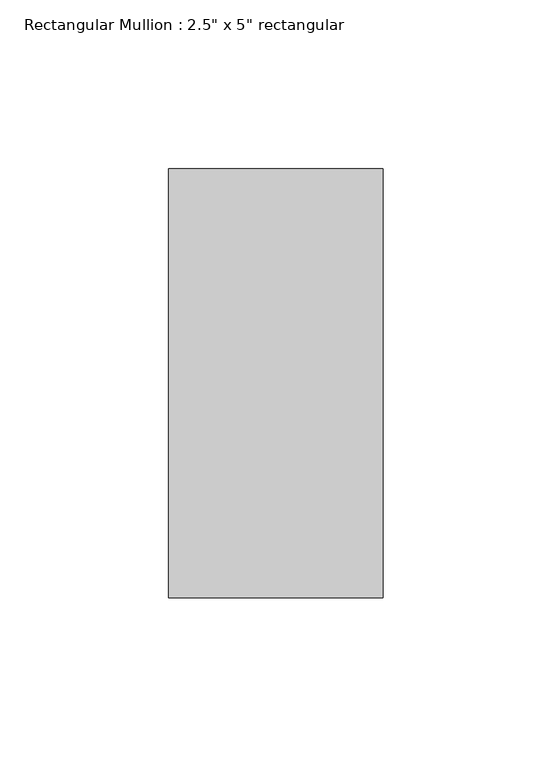
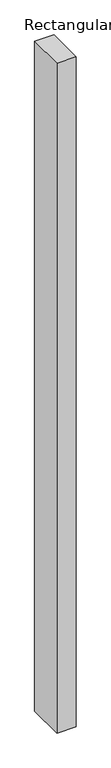
"""IFC4 building model written with IfcOpenShell, lengths in millimetres: member geometry."""

from ifc_helpers import new_model, si_unit, frame, origin, place, context, project, spatial, polyline, outline, extrude, source, transform, mapped, element, save


def member_a02723d6(model_context):
    return source(origin(), model_context, "Body", "SweptSolid", [
        extrude(outline(polyline([(0.0, 63.5), (0.0, -63.5), (-63.5, -63.5), (-63.5, 63.5), (0.0, 63.5)])), frame((0.0, 0.0, -2343.9308081), z_axis=(0.0, 0.0, 1.0), x_axis=(1.0, 0.0, 0.0)), (0.0, 0.0, 1.0), 2343.9308081),
    ])


if __name__ == "__main__":
    model = new_model("IFC4")
    model_context = context("Model", 3, world=origin())
    ifc_project = project(units=[si_unit("LENGTHUNIT", "METRE", prefix="MILLI")], contexts=[model_context])
    site = spatial("IfcSite", under=ifc_project)
    building = spatial("IfcBuilding", under=site)
    placement = place(None, origin())
    member_shape = member_a02723d6(model_context)
    element("IfcMember", 1, ObjectType="Rectangular Mullion : 2.5\" x 5\" rectangular", at=placement, inside=building, context=model_context, shape_type="MappedRepresentation", body=[
        mapped(member_shape, transform((0.0, 0.0, 0.0), x_axis=(1.0, 0.0, 0.0), y_axis=(0.0, 1.0, 0.0), z_axis=(0.0, 0.0, 1.0))),
    ])
    save(model, "model.ifc")

# Revit data of these elements
# Type "Rectangular Mullion : 2.5\" x 5\" rectangular"
#   built-in parameter 1007304 = 0.416667 (stored number, unit not read)
#   built-in parameter 1007301 = 0.104167 (stored number, unit not read)
#   built-in parameter 1007300 = 0.104167 (stored number, unit not read)
# Element 1 (IfcMember, "Rectangular Mullion : 2.5\" x 5\" rectangular")
#   Materials on its faces: "Aluminum"
# Materials
#   "Aluminum": class "Metal", colour RGB 247 247 247, transparency 0, Description = "Aluminum 6061", Cost = 0
